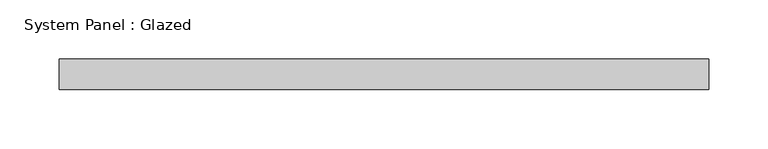
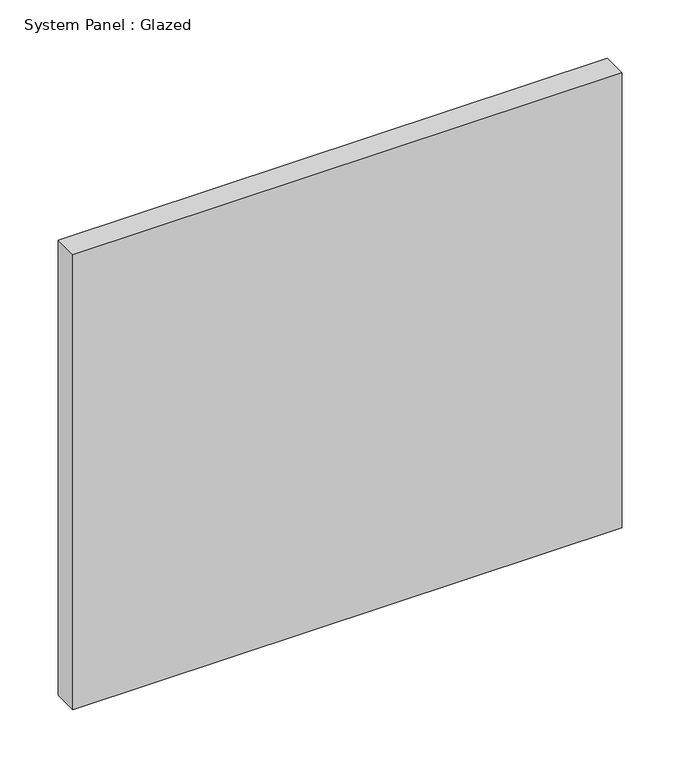
"""IFC4 building model written with IfcOpenShell, lengths in millimetres: plate geometry, System Panel : Glazed."""

from ifc_helpers import new_model, si_unit, origin, origin_with_axes, place, context, project, spatial, polyline, outline, extrude, source, transform, mapped, element, save


def system_panel_glazed_2ec405e4(model_context):
    return source(origin(), model_context, "Body", "SweptSolid", [
        extrude(outline(polyline([(273.05, 19.05), (-273.05, 19.05), (-273.05, 44.45), (273.05, 44.45), (273.05, 19.05)])), origin_with_axes(), (0.0, 0.0, 1.0), 478.3666667),
    ])


if __name__ == "__main__":
    model = new_model("IFC4")
    model_context = context("Model", 3, world=origin())
    ifc_project = project(units=[si_unit("LENGTHUNIT", "METRE", prefix="MILLI")], contexts=[model_context])
    site = spatial("IfcSite", under=ifc_project)
    building = spatial("IfcBuilding", under=site)
    placement = place(None, origin())
    system_panel_glazed_shape = system_panel_glazed_2ec405e4(model_context)
    element("IfcPlate", 1, ObjectType="System Panel : Glazed", at=placement, inside=building, context=model_context, shape_type="MappedRepresentation", body=[
        mapped(system_panel_glazed_shape, transform((0.0, 0.0, 0.0), x_axis=(1.0, 0.0, 0.0), y_axis=(0.0, 1.0, 0.0), z_axis=(0.0, 0.0, 1.0))),
    ])
    save(model, "model.ifc")

# Revit data of these elements
# Type "System Panel : Glazed"
#   Construction Type Id = "GSP4R"
#   Analytic Construction = "1/8 in Pilkington single glazing"
#   Visual Light Transmittance = 0.9
#   Solar Heat Gain Coefficient = 0.86
#   Heat Transfer Coefficient (U) = 1.18115 BTU/(h·ft²·°F)
#   Define Thermal Properties by = 1
# Element 1 (IfcPlate, "System Panel : Glazed")
#   Materials on its faces: "Glass"
# Materials
#   "Glass": class "Glass", colour RGB 0 128 192, transparency 0.75, Description = "Soda Lime Glass", Cost = 0
